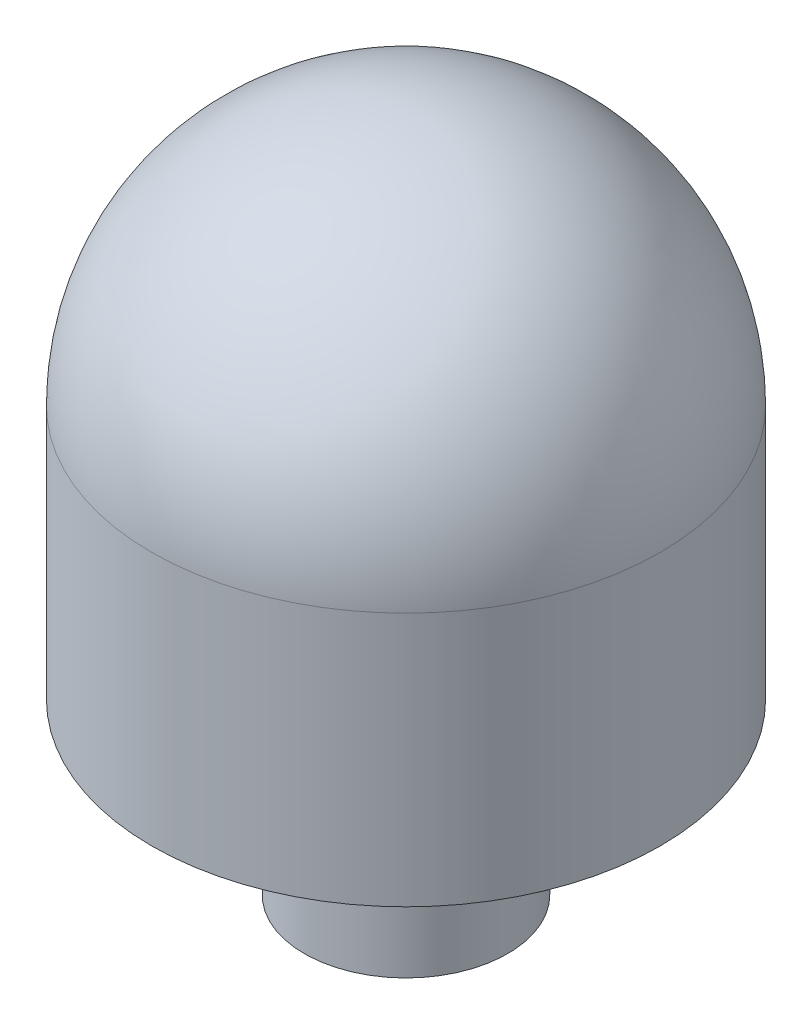
ISO-10303-21;
HEADER;
FILE_DESCRIPTION(('STEP AP214'),'2;1');
FILE_NAME('part.step','',(''),(''),'','','');
FILE_SCHEMA(('AUTOMOTIVE_DESIGN { 1 0 10303 214 1 1 1 1 }'));
ENDSEC;
DATA;
#1=APPLICATION_CONTEXT('core data for automotive mechanical design processes');
#2=APPLICATION_PROTOCOL_DEFINITION('international standard','automotive_design',2000,#1);
#3=PRODUCT_CONTEXT('',#1,'mechanical');
#4=PRODUCT('Part','Part','',(#3));
#5=PRODUCT_RELATED_PRODUCT_CATEGORY('part','',(#4));
#6=PRODUCT_DEFINITION_FORMATION('','',#4);
#7=PRODUCT_DEFINITION_CONTEXT('part definition',#1,'design');
#8=PRODUCT_DEFINITION('design','',#6,#7);
#9=PRODUCT_DEFINITION_SHAPE('','',#8);
#10=(LENGTH_UNIT() NAMED_UNIT(*) SI_UNIT(.MILLI.,.METRE.));
#11=(NAMED_UNIT(*) PLANE_ANGLE_UNIT() SI_UNIT($,.RADIAN.));
#12=(NAMED_UNIT(*) SI_UNIT($,.STERADIAN.) SOLID_ANGLE_UNIT());
#13=UNCERTAINTY_MEASURE_WITH_UNIT(LENGTH_MEASURE(1.E-05),#10,'distance_accuracy_value','');
#14=(GEOMETRIC_REPRESENTATION_CONTEXT(3) GLOBAL_UNCERTAINTY_ASSIGNED_CONTEXT((#13)) GLOBAL_UNIT_ASSIGNED_CONTEXT((#10,
#11,#12)) REPRESENTATION_CONTEXT('',''));
#15=CARTESIAN_POINT('',(0.,0.,0.));
#16=DIRECTION('',(0.,0.,1.));
#17=DIRECTION('',(1.,0.,0.));
#18=AXIS2_PLACEMENT_3D('',#15,#16,#17);
#19=CARTESIAN_POINT('',(0.,0.,0.));
#20=DIRECTION('',(0.,1.,0.));
#21=DIRECTION('',(-1.,0.,0.));
#22=AXIS2_PLACEMENT_3D('',#19,#20,#21);
#23=PLANE('',#22);
#24=CARTESIAN_POINT('',(0.,0.,0.));
#25=DIRECTION('',(0.,1.,0.));
#26=DIRECTION('',(-1.,0.,0.));
#27=AXIS2_PLACEMENT_3D('',#24,#25,#26);
#28=CIRCLE('',#27,6.);
#29=CARTESIAN_POINT('',(-6.,0.,0.));
#30=VERTEX_POINT('',#29);
#31=EDGE_CURVE('E10',#30,#30,#28,.T.);
#32=ORIENTED_EDGE('',*,*,#31,.F.);
#33=EDGE_LOOP('',(#32));
#34=FACE_BOUND('',#33,.T.);
#35=ADVANCED_FACE('F40',(#34),#23,.F.);
#36=CARTESIAN_POINT('',(0.,40.,0.));
#37=DIRECTION('',(0.,1.,0.));
#38=DIRECTION('',(-1.,0.,0.));
#39=AXIS2_PLACEMENT_3D('',#36,#37,#38);
#40=CYLINDRICAL_SURFACE('',#39,6.);
#41=CARTESIAN_POINT('',(0.,10.,0.));
#42=DIRECTION('',(0.,1.,0.));
#43=DIRECTION('',(-1.,0.,0.));
#44=AXIS2_PLACEMENT_3D('',#41,#42,#43);
#45=CIRCLE('',#44,6.);
#46=CARTESIAN_POINT('',(-6.,10.,0.));
#47=VERTEX_POINT('',#46);
#48=EDGE_CURVE('E43',#47,#47,#45,.T.);
#49=ORIENTED_EDGE('',*,*,#48,.F.);
#50=EDGE_LOOP('',(#49));
#51=FACE_BOUND('',#50,.T.);
#52=ORIENTED_EDGE('',*,*,#31,.T.);
#53=EDGE_LOOP('',(#52));
#54=FACE_BOUND('',#53,.T.);
#55=ADVANCED_FACE('F67',(#51,#54),#40,.T.);
#56=CARTESIAN_POINT('',(6.,10.,0.));
#57=DIRECTION('',(0.,1.,0.));
#58=DIRECTION('',(-1.,0.,0.));
#59=AXIS2_PLACEMENT_3D('',#56,#57,#58);
#60=PLANE('',#59);
#61=CARTESIAN_POINT('',(0.,10.,0.));
#62=DIRECTION('',(0.,1.,0.));
#63=DIRECTION('',(-1.,0.,0.));
#64=AXIS2_PLACEMENT_3D('',#61,#62,#63);
#65=CIRCLE('',#64,15.);
#66=CARTESIAN_POINT('',(-15.,10.,0.));
#67=VERTEX_POINT('',#66);
#68=EDGE_CURVE('E50',#67,#67,#65,.T.);
#69=ORIENTED_EDGE('',*,*,#68,.F.);
#70=EDGE_LOOP('',(#69));
#71=FACE_BOUND('',#70,.T.);
#72=ORIENTED_EDGE('',*,*,#48,.T.);
#73=EDGE_LOOP('',(#72));
#74=FACE_BOUND('',#73,.T.);
#75=ADVANCED_FACE('F65',(#71,#74),#60,.F.);
#76=CARTESIAN_POINT('',(0.,40.,0.));
#77=DIRECTION('',(0.,1.,0.));
#78=DIRECTION('',(-1.,0.,0.));
#79=AXIS2_PLACEMENT_3D('',#76,#77,#78);
#80=CYLINDRICAL_SURFACE('',#79,15.);
#81=CARTESIAN_POINT('',(0.,25.,0.));
#82=DIRECTION('',(0.,1.,0.));
#83=DIRECTION('',(-1.,0.,0.));
#84=AXIS2_PLACEMENT_3D('',#81,#82,#83);
#85=CIRCLE('',#84,15.);
#86=CARTESIAN_POINT('',(-15.,25.,0.));
#87=VERTEX_POINT('',#86);
#88=EDGE_CURVE('E51',#87,#87,#85,.T.);
#89=ORIENTED_EDGE('',*,*,#88,.F.);
#90=EDGE_LOOP('',(#89));
#91=FACE_BOUND('',#90,.T.);
#92=ORIENTED_EDGE('',*,*,#68,.T.);
#93=EDGE_LOOP('',(#92));
#94=FACE_BOUND('',#93,.T.);
#95=ADVANCED_FACE('F56',(#91,#94),#80,.T.);
#96=CARTESIAN_POINT('',(0.,25.,0.));
#97=DIRECTION('',(0.,1.,0.));
#98=DIRECTION('',(1.,0.,0.));
#99=AXIS2_PLACEMENT_3D('',#96,#97,#98);
#100=SPHERICAL_SURFACE('',#99,15.);
#101=ORIENTED_EDGE('',*,*,#88,.T.);
#102=EDGE_LOOP('',(#101));
#103=FACE_BOUND('',#102,.T.);
#104=ADVANCED_FACE('F60',(#103),#100,.T.);
#105=CLOSED_SHELL('',(#35,#55,#75,#95,#104));
#106=MANIFOLD_SOLID_BREP('B2',#105);
#107=ADVANCED_BREP_SHAPE_REPRESENTATION('',(#18,#106),#14);
#108=SHAPE_DEFINITION_REPRESENTATION(#9,#107);
ENDSEC;
END-ISO-10303-21;
